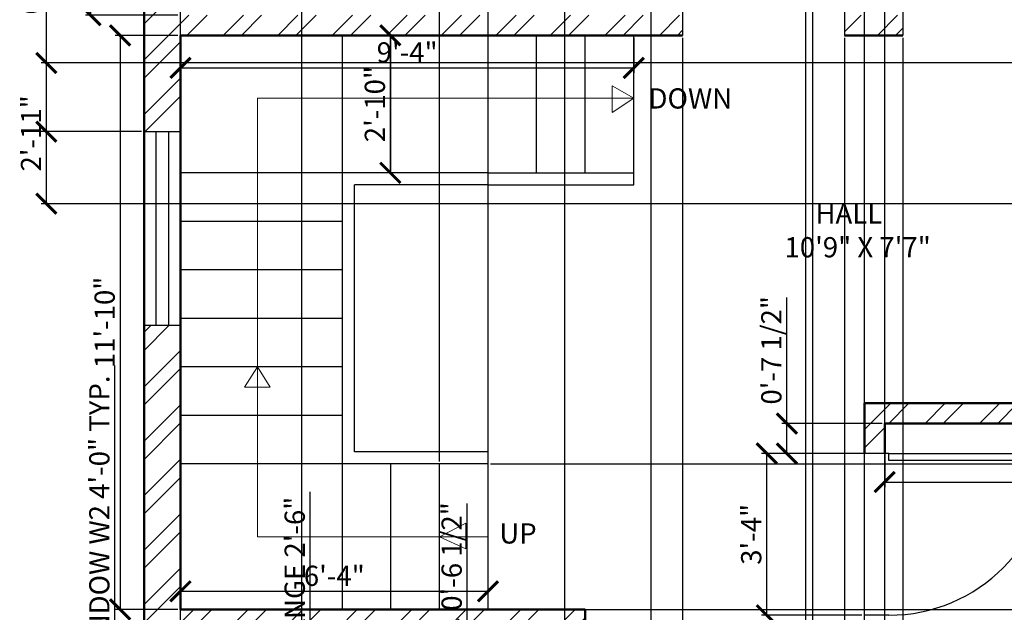
# Model space of a CAD drawing. Units: inches. Extents: x 683 to 1274, y 1901 to 2385.
# Tile 2 of 5: x 687 to 930, y 2049 to 2196. Entities that reach past the tile are written whole.
import ezdxf

# ---------------------------------------------------------------- set-up
doc = ezdxf.new("R2010")
doc.units = ezdxf.units.IN
for name, color, linetype, lineweight in [('A-ANNO-SYMB', 1, 'Continuous', 18), ('A-AREA-IDEN', 3, 'Continuous', 25), ('A-FLOR-STRS', 7, 'Continuous', 25), ('A-WALL-PATT', 8, 'Continuous', 13), ('DIM', 3, 'Continuous', 18), ('DOORS', 4, 'Continuous', 25), ('TEXT', 1, 'Continuous', 25), ('walls', 6, 'Continuous', 50), ('WINDOWS', 30, 'Continuous', 25)]:
    doc.layers.add(name, color=color, linetype=linetype, lineweight=lineweight)
doc.styles.get("Standard").update_dxf_attribs({"font": 'arial.ttf'})
doc.dimstyles.new('ISO-25', dxfattribs={"dimtxt": 5, "dimasz": 5, "dimexe": 1.25, "dimexo": 0.625, "dimtad": 1, "dimdec": 1, "dimlunit": 4, "dimtxsty": 'Standard', "dimblk": 'ARCHTICK', "dimcen": 2.5, "dimadec": 0, "dimazin": 0, "dimtfac": 1, "dimtdec": 1, "dimtmove": 0, "dimatfit": 3, "dimfxl": 1, "dimarcsym": 0})

# ---------------------------------------------------------------- blocks, each defined once
blk = doc.blocks.new('_ArchTick')
at = {"color": 0, "linetype": 'ByBlock', "const_width": 0.15}
blk.add_lwpolyline([(-0.5, -0.5), (0.5, 0.5)], dxfattribs=at)
blk = doc.blocks.new('*D8')
at = {"layer": 'Defpoints', "color": 0, "transparency": 16777216}
for p in [(900.42, 2095.78), (1020.42, 2095.78), (1020.42, 2081.28)]:
    blk.add_point(p, dxfattribs=at)
at = {"layer": 'DIM', "color": 0, "lineweight": -2, "transparency": 16777216}
for p, q in [((900.42, 2095.16), (900.42, 2080.03)), ((1020.42, 2095.16), (1020.42, 2080.03)), ((900.42, 2081.28), (1020.42, 2081.28))]:
    blk.add_line(p, q, dxfattribs=at)
at = {"layer": 'DIM', "color": 0, "lineweight": -2, "transparency": 16777216, "xscale": 5, "yscale": 5, "zscale": 5, "rotation": 180}
blk.add_blockref('_ArchTick', (900.42, 2081.28), dxfattribs=at)
at = {"layer": 'DIM', "color": 0, "lineweight": -2, "transparency": 16777216, "xscale": 5, "yscale": 5, "zscale": 5}
blk.add_blockref('_ArchTick', (1020.42, 2081.28), dxfattribs=at)
at = {"layer": 'DIM', "color": 0, "transparency": 16777216, "insert": (960.42, 2084.46), "char_height": 5, "attachment_point": 5}
blk.add_mtext("10'", dxfattribs=at)
blk = doc.blocks.new('*D12')
at = {"layer": 'Defpoints', "color": 0, "transparency": 16777216}
for p in [(726.42, 2191.78), (838.42, 2191.78), (838.42, 2183.74)]:
    blk.add_point(p, dxfattribs=at)
at = {"layer": 'DIM', "color": 0, "lineweight": -2, "transparency": 16777216}
for p, q in [((726.42, 2191.16), (726.42, 2182.49)), ((838.42, 2191.16), (838.42, 2182.49)), ((726.42, 2183.74), (838.42, 2183.74))]:
    blk.add_line(p, q, dxfattribs=at)
at = {"layer": 'DIM', "color": 0, "lineweight": -2, "transparency": 16777216, "xscale": 5, "yscale": 5, "zscale": 5, "rotation": 180}
blk.add_blockref('_ArchTick', (726.42, 2183.74), dxfattribs=at)
at = {"layer": 'DIM', "color": 0, "lineweight": -2, "transparency": 16777216, "xscale": 5, "yscale": 5, "zscale": 5}
blk.add_blockref('_ArchTick', (838.42, 2183.74), dxfattribs=at)
at = {"layer": 'DIM', "color": 0, "transparency": 16777216, "insert": (782.42, 2186.92), "char_height": 5, "attachment_point": 5}
blk.add_mtext('9\'-4"', dxfattribs=at)
blk = doc.blocks.new('*D13')
at = {"layer": 'Defpoints', "color": 0, "transparency": 16777216}
for p in [(802.42, 2054.27), (726.42, 2049.78), (802.42, 2049.78)]:
    blk.add_point(p, dxfattribs=at)
at = {"layer": 'DIM', "color": 0, "lineweight": -2, "transparency": 16777216}
for p, q in [((726.42, 2050.41), (726.42, 2055.52)), ((726.42, 2054.27), (802.42, 2054.27)), ((802.42, 2050.41), (802.42, 2055.52))]:
    blk.add_line(p, q, dxfattribs=at)
at = {"layer": 'DIM', "color": 0, "lineweight": -2, "transparency": 16777216, "xscale": 5, "yscale": 5, "zscale": 5, "rotation": 180}
blk.add_blockref('_ArchTick', (726.42, 2054.27), dxfattribs=at)
at = {"layer": 'DIM', "color": 0, "lineweight": -2, "transparency": 16777216, "xscale": 5, "yscale": 5, "zscale": 5}
blk.add_blockref('_ArchTick', (802.42, 2054.27), dxfattribs=at)
at = {"layer": 'DIM', "color": 0, "transparency": 16777216, "insert": (764.42, 2057.45), "char_height": 5, "attachment_point": 5}
blk.add_mtext('6\'-4"', dxfattribs=at)
blk = doc.blocks.new('W2')
at = {"layer": 'WINDOWS'}
for p, q in [((1126.75, 2245.25), (1135.75, 2245.25)), ((1126.75, 2197.25), (1126.75, 2245.25)), ((1129.75, 2197.25), (1129.75, 2245.25)), ((1132.75, 2245.25), (1132.75, 2197.25)), ((1135.75, 2245.25), (1135.75, 2197.25)), ((1135.75, 2197.25), (1126.75, 2197.25))]:
    blk.add_line(p, q, dxfattribs=at)
blk = doc.blocks.new('*U18')
for p, q in [((0, 0), (0, -6)), ((40, 0), (40, -6))]:
    blk.add_line(p, q)
blk.add_lwpolyline([(0, 0), (0, 40), (1.75, 40), (1.75, 0)], close=True)
blk.add_arc((0, 0), 40, 0, 90)
blk = doc.blocks.new('*D19')
at = {"layer": 'Defpoints', "color": 0, "transparency": 16777216}
for p in [(726.42, 2328.78), (704.19, 2196.78), (726.42, 2196.78)]:
    blk.add_point(p, dxfattribs=at)
at = {"layer": 'DIM', "color": 0, "lineweight": -2, "transparency": 16777216}
for p, q in [((725.79, 2328.78), (702.94, 2328.78)), ((704.19, 2328.78), (704.19, 2196.78)), ((725.79, 2196.78), (702.94, 2196.78))]:
    blk.add_line(p, q, dxfattribs=at)
at = {"layer": 'DIM', "color": 0, "lineweight": -2, "transparency": 16777216, "xscale": 5, "yscale": 5, "zscale": 5}
for p, rotation in [((704.19, 2328.78), 90), ((704.19, 2196.78), 270)]:
    blk.add_blockref('_ArchTick', p, dxfattribs=dict(at, rotation=rotation))
at = {"layer": 'DIM', "color": 0, "transparency": 16777216, "insert": (701.05, 2262.78), "char_height": 5, "attachment_point": 5, "rotation": 90}
blk.add_mtext("11'", dxfattribs=at)
blk = doc.blocks.new('*D23')
at = {"layer": 'Defpoints', "color": 0, "transparency": 16777216}
for p in [(726.42, 2191.78), (711.49, 2049.78), (726.42, 2049.78)]:
    blk.add_point(p, dxfattribs=at)
at = {"layer": 'DIM', "color": 0, "lineweight": -2, "transparency": 16777216}
for p, q in [((725.79, 2191.78), (710.24, 2191.78)), ((711.49, 2191.78), (711.49, 2049.78)), ((725.79, 2049.78), (710.24, 2049.78))]:
    blk.add_line(p, q, dxfattribs=at)
at = {"layer": 'DIM', "color": 0, "lineweight": -2, "transparency": 16777216, "xscale": 5, "yscale": 5, "zscale": 5}
for p, rotation in [((711.49, 2191.78), 90), ((711.49, 2049.78), 270)]:
    blk.add_blockref('_ArchTick', p, dxfattribs=dict(at, rotation=rotation))
at = {"layer": 'DIM', "color": 0, "transparency": 16777216, "insert": (708.32, 2120.78), "char_height": 5, "attachment_point": 5, "rotation": 90}
blk.add_mtext('11\'-10"', dxfattribs=at)
blk = doc.blocks.new('*D29')
at = {"layer": 'Defpoints', "color": 0, "transparency": 16777216}
for p in [(710.22, 2028.18), (717.42, 2028.18), (717.42, 1980.18)]:
    blk.add_point(p, dxfattribs=at)
at = {"layer": 'DIM', "color": 0, "lineweight": -2, "transparency": 16777216}
for p, q in [((710.22, 2028.18), (710.22, 2110.12)), ((716.79, 2028.18), (708.97, 2028.18)), ((710.22, 1980.18), (710.22, 2028.18)), ((716.79, 1980.18), (708.97, 1980.18))]:
    blk.add_line(p, q, dxfattribs=at)
at = {"layer": 'DIM', "color": 0, "lineweight": -2, "transparency": 16777216, "xscale": 5, "yscale": 5, "zscale": 5}
for p, rotation in [((710.22, 2028.18), 90), ((710.22, 1980.18), 270)]:
    blk.add_blockref('_ArchTick', p, dxfattribs=dict(at, rotation=rotation))
at = {"layer": 'DIM', "color": 0, "transparency": 16777216, "insert": (707.01, 2071.65), "char_height": 5, "attachment_point": 5, "rotation": 90}
blk.add_mtext('WINDOW W2 4\'-0" TYP.', dxfattribs=at)
blk = doc.blocks.new('*D33')
at = {"layer": 'Defpoints', "color": 0, "transparency": 16777216}
for p in [(754, 2032.78), (758.5, 2032.78), (754, 2002.78)]:
    blk.add_point(p, dxfattribs=at)
at = {"layer": 'DIM', "color": 0, "lineweight": -2, "transparency": 16777216}
for p, q in [((758.5, 2032.78), (758.5, 2078.84)), ((754.63, 2032.78), (759.75, 2032.78)), ((758.5, 2002.78), (758.5, 2032.78)), ((754.63, 2002.78), (759.75, 2002.78))]:
    blk.add_line(p, q, dxfattribs=at)
at = {"layer": 'DIM', "color": 0, "lineweight": -2, "transparency": 16777216, "xscale": 5, "yscale": 5, "zscale": 5}
for p, rotation in [((758.5, 2032.78), 90), ((758.5, 2002.78), 270)]:
    blk.add_blockref('_ArchTick', p, dxfattribs=dict(at, rotation=rotation))
at = {"layer": 'DIM', "color": 0, "transparency": 16777216, "insert": (755.29, 2058.31), "char_height": 5, "attachment_point": 5, "rotation": 90}
blk.add_mtext('RANGE 2\'-6"', dxfattribs=at)
blk = doc.blocks.new('*D39')
at = {"layer": 'Defpoints', "color": 0, "transparency": 16777216}
for p in [(900.42, 2361.93), (821.42, 1929.78), (900.42, 1929.78)]:
    blk.add_point(p, dxfattribs=at)
at = {"layer": 'DIM', "color": 0, "lineweight": -2, "transparency": 16777216}
for p, q in [((821.42, 1930.41), (821.42, 2363.18)), ((900.42, 1930.41), (900.42, 2363.18)), ((821.42, 2361.93), (900.42, 2361.93))]:
    blk.add_line(p, q, dxfattribs=at)
at = {"layer": 'DIM', "color": 0, "lineweight": -2, "transparency": 16777216, "xscale": 5, "yscale": 5, "zscale": 5, "rotation": 180}
blk.add_blockref('_ArchTick', (821.42, 2361.93), dxfattribs=at)
at = {"layer": 'DIM', "color": 0, "lineweight": -2, "transparency": 16777216, "xscale": 5, "yscale": 5, "zscale": 5}
blk.add_blockref('_ArchTick', (900.42, 2361.93), dxfattribs=at)
at = {"layer": 'DIM', "color": 0, "transparency": 16777216, "insert": (860.92, 2365.11), "char_height": 5, "attachment_point": 5}
blk.add_mtext('6\'-7"', dxfattribs=at)
blk = doc.blocks.new('*D43')
at = {"layer": 'Defpoints', "color": 0, "transparency": 16777216}
for p in [(693.27, 2184.95), (967.42, 2184.95), (967.42, 2150.14)]:
    blk.add_point(p, dxfattribs=at)
at = {"layer": 'DIM', "color": 0, "lineweight": -2, "transparency": 16777216}
for p, q in [((966.79, 2184.95), (692.02, 2184.95)), ((693.27, 2150.14), (693.27, 2184.95)), ((966.79, 2150.14), (692.02, 2150.14))]:
    blk.add_line(p, q, dxfattribs=at)
at = {"layer": 'DIM', "color": 0, "lineweight": -2, "transparency": 16777216, "xscale": 5, "yscale": 5, "zscale": 5}
for p, rotation in [((693.27, 2184.95), 90), ((693.27, 2150.14), 270)]:
    blk.add_blockref('_ArchTick', p, dxfattribs=dict(at, rotation=rotation))
at = {"layer": 'DIM', "color": 0, "transparency": 16777216, "insert": (690.13, 2167.54), "char_height": 5, "attachment_point": 5, "rotation": 90}
blk.add_mtext('2\'-11"', dxfattribs=at)
blk = doc.blocks.new('*D44')
at = {"layer": 'Defpoints', "color": 0, "transparency": 16777216}
for p in [(882.7, 2361.93), (842.7, 1953.78), (882.7, 1953.78)]:
    blk.add_point(p, dxfattribs=at)
at = {"layer": 'DIM', "color": 0, "lineweight": -2, "transparency": 16777216}
for p, q in [((842.7, 1954.41), (842.7, 2363.18)), ((882.7, 1954.41), (882.7, 2363.18)), ((842.7, 2361.93), (882.7, 2361.93))]:
    blk.add_line(p, q, dxfattribs=at)
at = {"layer": 'DIM', "color": 0, "lineweight": -2, "transparency": 16777216, "xscale": 5, "yscale": 5, "zscale": 5, "rotation": 180}
blk.add_blockref('_ArchTick', (842.7, 2361.93), dxfattribs=at)
at = {"layer": 'DIM', "color": 0, "lineweight": -2, "transparency": 16777216, "xscale": 5, "yscale": 5, "zscale": 5}
blk.add_blockref('_ArchTick', (882.7, 2361.93), dxfattribs=at)
at = {"layer": 'DIM', "color": 0, "transparency": 16777216, "insert": (862.7, 2365.11), "char_height": 5, "attachment_point": 5}
blk.add_mtext('3\'-4"', dxfattribs=at)
blk = doc.blocks.new('*D45')
at = {"layer": 'Defpoints', "color": 0, "transparency": 16777216}
for p in [(850.48, 2191.78), (890.48, 2191.78), (890.48, 1905.63)]:
    blk.add_point(p, dxfattribs=at)
at = {"layer": 'DIM', "color": 0, "lineweight": -2, "transparency": 16777216}
for p, q in [((850.48, 2191.16), (850.48, 1904.38)), ((890.48, 2191.16), (890.48, 1904.38)), ((850.48, 1905.63), (890.48, 1905.63))]:
    blk.add_line(p, q, dxfattribs=at)
at = {"layer": 'DIM', "color": 0, "lineweight": -2, "transparency": 16777216, "xscale": 5, "yscale": 5, "zscale": 5, "rotation": 180}
blk.add_blockref('_ArchTick', (850.48, 1905.63), dxfattribs=at)
at = {"layer": 'DIM', "color": 0, "lineweight": -2, "transparency": 16777216, "xscale": 5, "yscale": 5, "zscale": 5}
blk.add_blockref('_ArchTick', (890.48, 1905.63), dxfattribs=at)
at = {"layer": 'DIM', "color": 0, "transparency": 16777216, "insert": (870.48, 1908.81), "char_height": 5, "attachment_point": 5}
blk.add_mtext('3\'-4"', dxfattribs=at)
blk = doc.blocks.new('*D46')
at = {"layer": 'Defpoints', "color": 0, "transparency": 16777216}
for p in [(904.89, 2191.78), (944.89, 2191.78), (944.89, 1905.63)]:
    blk.add_point(p, dxfattribs=at)
at = {"layer": 'DIM', "color": 0, "lineweight": -2, "transparency": 16777216}
for p, q in [((904.89, 2191.16), (904.89, 1904.38)), ((944.89, 2191.16), (944.89, 1904.38)), ((904.89, 1905.63), (944.89, 1905.63))]:
    blk.add_line(p, q, dxfattribs=at)
at = {"layer": 'DIM', "color": 0, "lineweight": -2, "transparency": 16777216, "xscale": 5, "yscale": 5, "zscale": 5, "rotation": 180}
blk.add_blockref('_ArchTick', (904.89, 1905.63), dxfattribs=at)
at = {"layer": 'DIM', "color": 0, "lineweight": -2, "transparency": 16777216, "xscale": 5, "yscale": 5, "zscale": 5}
blk.add_blockref('_ArchTick', (944.89, 1905.63), dxfattribs=at)
at = {"layer": 'DIM', "color": 0, "transparency": 16777216, "insert": (924.89, 1908.81), "char_height": 5, "attachment_point": 5}
blk.add_mtext('3\'-4"', dxfattribs=at)
blk = doc.blocks.new('*D47')
at = {"layer": 'Defpoints', "color": 0, "transparency": 16777216}
for p in [(871.27, 2088.36), (895.42, 2088.36), (895.42, 2048.36)]:
    blk.add_point(p, dxfattribs=at)
at = {"layer": 'DIM', "color": 0, "lineweight": -2, "transparency": 16777216}
for p, q in [((894.79, 2088.36), (870.02, 2088.36)), ((871.27, 2048.36), (871.27, 2088.36)), ((894.79, 2048.36), (870.02, 2048.36))]:
    blk.add_line(p, q, dxfattribs=at)
at = {"layer": 'DIM', "color": 0, "lineweight": -2, "transparency": 16777216, "xscale": 5, "yscale": 5, "zscale": 5}
for p, rotation in [((871.27, 2088.36), 90), ((871.27, 2048.36), 270)]:
    blk.add_blockref('_ArchTick', p, dxfattribs=dict(at, rotation=rotation))
at = {"layer": 'DIM', "color": 0, "transparency": 16777216, "insert": (868.09, 2068.36), "char_height": 5, "attachment_point": 5, "rotation": 90}
blk.add_mtext('3\'-4"', dxfattribs=at)
blk = doc.blocks.new('*D48')
at = {"layer": 'Defpoints', "color": 0, "transparency": 16777216}
for p in [(778.27, 2191.78), (802.42, 2191.78), (802.42, 2157.78)]:
    blk.add_point(p, dxfattribs=at)
at = {"layer": 'DIM', "color": 0, "lineweight": -2, "transparency": 16777216}
for p, q in [((801.79, 2191.78), (777.02, 2191.78)), ((778.27, 2157.78), (778.27, 2191.78)), ((801.79, 2157.78), (777.02, 2157.78))]:
    blk.add_line(p, q, dxfattribs=at)
at = {"layer": 'DIM', "color": 0, "lineweight": -2, "transparency": 16777216, "xscale": 5, "yscale": 5, "zscale": 5}
for p, rotation in [((778.27, 2191.78), 90), ((778.27, 2157.78), 270)]:
    blk.add_blockref('_ArchTick', p, dxfattribs=dict(at, rotation=rotation))
at = {"layer": 'DIM', "color": 0, "transparency": 16777216, "insert": (775.09, 2174.78), "char_height": 5, "attachment_point": 5, "rotation": 90}
blk.add_mtext('2\'-10"', dxfattribs=at)
blk = doc.blocks.new('*D49')
at = {"layer": 'Defpoints', "color": 0, "transparency": 16777216}
for p in [(802.42, 2085.78), (1053.57, 2085.78), (802.42, 2049.78)]:
    blk.add_point(p, dxfattribs=at)
at = {"layer": 'DIM', "color": 0, "lineweight": -2, "transparency": 16777216}
for p, q in [((803.04, 2085.78), (1054.82, 2085.78)), ((1053.57, 2049.78), (1053.57, 2085.78)), ((803.04, 2049.78), (1054.82, 2049.78))]:
    blk.add_line(p, q, dxfattribs=at)
at = {"layer": 'DIM', "color": 0, "lineweight": -2, "transparency": 16777216, "xscale": 5, "yscale": 5, "zscale": 5}
for p, rotation in [((1053.57, 2085.78), 90), ((1053.57, 2049.78), 270)]:
    blk.add_blockref('_ArchTick', p, dxfattribs=dict(at, rotation=rotation))
at = {"layer": 'DIM', "color": 0, "transparency": 16777216, "insert": (1050.39, 2067.78), "char_height": 5, "attachment_point": 5, "rotation": 90}
blk.add_mtext('3\'-0"', dxfattribs=at)
blk = doc.blocks.new('*D50')
at = {"layer": 'Defpoints', "color": 0, "transparency": 16777216}
for p in [(802.42, 2361.93), (790.42, 2085.78), (802.42, 2085.78)]:
    blk.add_point(p, dxfattribs=at)
at = {"layer": 'DIM', "color": 0, "lineweight": -2, "transparency": 16777216}
for p, q in [((790.42, 2086.41), (790.42, 2363.18)), ((802.42, 2086.41), (802.42, 2363.18)), ((790.42, 2361.93), (802.42, 2361.93)), ((802.42, 2361.93), (821.49, 2361.93))]:
    blk.add_line(p, q, dxfattribs=at)
at = {"layer": 'DIM', "color": 0, "lineweight": -2, "transparency": 16777216, "xscale": 5, "yscale": 5, "zscale": 5, "rotation": 180}
blk.add_blockref('_ArchTick', (790.42, 2361.93), dxfattribs=at)
at = {"layer": 'DIM', "color": 0, "lineweight": -2, "transparency": 16777216, "xscale": 5, "yscale": 5, "zscale": 5}
blk.add_blockref('_ArchTick', (802.42, 2361.93), dxfattribs=at)
at = {"layer": 'DIM', "color": 0, "transparency": 16777216, "insert": (814.45, 2365.11), "char_height": 5, "attachment_point": 5}
blk.add_mtext('1\'-0"', dxfattribs=at)
blk = doc.blocks.new('*D55')
at = {"layer": 'Defpoints', "color": 0, "transparency": 16777216}
for p in [(693.27, 2240.95), (717.42, 2240.95), (717.42, 2167.98)]:
    blk.add_point(p, dxfattribs=at)
at = {"layer": 'DIM', "color": 0, "lineweight": -2, "transparency": 16777216}
for p, q in [((716.79, 2240.95), (692.02, 2240.95)), ((693.27, 2167.98), (693.27, 2240.95)), ((716.79, 2167.98), (692.02, 2167.98))]:
    blk.add_line(p, q, dxfattribs=at)
at = {"layer": 'DIM', "color": 0, "lineweight": -2, "transparency": 16777216, "xscale": 5, "yscale": 5, "zscale": 5}
for p, rotation in [((693.27, 2240.95), 90), ((693.27, 2167.98), 270)]:
    blk.add_blockref('_ArchTick', p, dxfattribs=dict(at, rotation=rotation))
at = {"layer": 'DIM', "color": 0, "transparency": 16777216, "insert": (690.09, 2204.46), "char_height": 5, "attachment_point": 5, "rotation": 90}
blk.add_mtext('6\'-1"', dxfattribs=at)
blk = doc.blocks.new('*D58')
at = {"layer": 'Defpoints', "color": 0, "transparency": 16777216}
for p in [(756.42, 2361.93), (726.42, 2044.78), (756.42, 2044.78)]:
    blk.add_point(p, dxfattribs=at)
at = {"layer": 'DIM', "color": 0, "lineweight": -2, "transparency": 16777216}
for p, q in [((726.42, 2045.41), (726.42, 2363.18)), ((756.42, 2045.41), (756.42, 2363.18)), ((726.42, 2361.93), (756.42, 2361.93))]:
    blk.add_line(p, q, dxfattribs=at)
at = {"layer": 'DIM', "color": 0, "lineweight": -2, "transparency": 16777216, "xscale": 5, "yscale": 5, "zscale": 5, "rotation": 180}
blk.add_blockref('_ArchTick', (726.42, 2361.93), dxfattribs=at)
at = {"layer": 'DIM', "color": 0, "lineweight": -2, "transparency": 16777216, "xscale": 5, "yscale": 5, "zscale": 5}
blk.add_blockref('_ArchTick', (756.42, 2361.93), dxfattribs=at)
at = {"layer": 'DIM', "color": 0, "transparency": 16777216, "insert": (741.42, 2365.11), "char_height": 5, "attachment_point": 5}
blk.add_mtext('2\'-6"', dxfattribs=at)
blk = doc.blocks.new('*D61')
at = {"layer": 'Defpoints', "color": 0, "transparency": 16777216}
for p in [(895.42, 2361.93), (880.95, 1962.78), (895.42, 1962.78)]:
    blk.add_point(p, dxfattribs=at)
at = {"layer": 'DIM', "color": 0, "lineweight": -2, "transparency": 16777216}
for p, q in [((880.95, 1963.41), (880.95, 2363.18)), ((895.42, 1963.41), (895.42, 2363.18)), ((880.95, 2361.93), (895.42, 2361.93)), ((895.42, 2361.93), (926.14, 2361.93))]:
    blk.add_line(p, q, dxfattribs=at)
at = {"layer": 'DIM', "color": 0, "lineweight": -2, "transparency": 16777216, "xscale": 5, "yscale": 5, "zscale": 5, "rotation": 180}
blk.add_blockref('_ArchTick', (880.95, 2361.93), dxfattribs=at)
at = {"layer": 'DIM', "color": 0, "lineweight": -2, "transparency": 16777216, "xscale": 5, "yscale": 5, "zscale": 5}
blk.add_blockref('_ArchTick', (895.42, 2361.93), dxfattribs=at)
at = {"layer": 'DIM', "color": 0, "transparency": 16777216, "insert": (913.28, 2365.14), "char_height": 5, "attachment_point": 5}
blk.add_mtext('1\'-2 1/2"', dxfattribs=at)
blk = doc.blocks.new('*D65')
at = {"layer": 'Defpoints', "color": 0, "transparency": 16777216}
for p in [(876.27, 2095.78), (900.42, 2095.78), (900.42, 2088.36)]:
    blk.add_point(p, dxfattribs=at)
at = {"layer": 'DIM', "color": 0, "lineweight": -2, "transparency": 16777216}
for p, q in [((876.27, 2095.78), (876.27, 2126.97)), ((899.79, 2095.78), (875.02, 2095.78)), ((876.27, 2088.36), (876.27, 2095.78)), ((899.79, 2088.36), (875.02, 2088.36))]:
    blk.add_line(p, q, dxfattribs=at)
at = {"layer": 'DIM', "color": 0, "lineweight": -2, "transparency": 16777216, "xscale": 5, "yscale": 5, "zscale": 5}
for p, rotation in [((876.27, 2095.78), 90), ((876.27, 2088.36), 270)]:
    blk.add_blockref('_ArchTick', p, dxfattribs=dict(at, rotation=rotation))
at = {"layer": 'DIM', "color": 0, "transparency": 16777216, "insert": (873.06, 2113.88), "char_height": 5, "attachment_point": 5, "rotation": 90}
blk.add_mtext('0\'-7 1/2"', dxfattribs=at)
blk = doc.blocks.new('*D66')
at = {"layer": 'Defpoints', "color": 0, "transparency": 16777216}
for p in [(797.27, 2044.78), (821.42, 2044.78), (821.42, 2038.04)]:
    blk.add_point(p, dxfattribs=at)
at = {"layer": 'DIM', "color": 0, "lineweight": -2, "transparency": 16777216}
for p, q in [((797.27, 2044.78), (797.27, 2075.97)), ((820.79, 2044.78), (796.02, 2044.78)), ((797.27, 2038.04), (797.27, 2044.78)), ((820.79, 2038.04), (796.02, 2038.04))]:
    blk.add_line(p, q, dxfattribs=at)
at = {"layer": 'DIM', "color": 0, "lineweight": -2, "transparency": 16777216, "xscale": 5, "yscale": 5, "zscale": 5}
for p, rotation in [((797.27, 2044.78), 90), ((797.27, 2038.04), 270)]:
    blk.add_blockref('_ArchTick', p, dxfattribs=dict(at, rotation=rotation))
at = {"layer": 'DIM', "color": 0, "transparency": 16777216, "insert": (794.06, 2062.88), "char_height": 5, "attachment_point": 5, "rotation": 90}
blk.add_mtext('0\'-6 1/2"', dxfattribs=at)

msp = doc.modelspace()

# ---------------------------------------------------------------- hatches: boundary and pattern name
at = {"layer": 'A-WALL-PATT'}
h = msp.add_hatch(dxfattribs=at)
h.set_pattern_fill('ANSI32', color=256)
h.paths.add_polyline_path([(717.42, 2337.78), (717.42, 2300.95), (726.42, 2300.95), (726.42, 2328.78), (895.42, 2328.78), (895.42, 2196.78), (890.48, 2196.78), (890.48, 2191.78), (904.89, 2191.78), (904.89, 2196.78), (900.42, 2196.78), (900.42, 2328.78), (1020.42, 2328.78), (1020.42, 2303.09), (1029.42, 2303.09), (1029.42, 2337.78)])
h.paths.add_polyline_path([(1020.42, 2196.78), (944.89, 2196.78), (944.89, 2191.78), (967.42, 2191.78), (967.42, 2184.95), (972.42, 2184.95), (972.42, 2191.78), (1020.42, 2191.78), (1020.42, 2129.51), (1029.42, 2129.51), (1029.42, 2243.09), (1020.42, 2243.09)])
h.paths.add_polyline_path([(1029.42, 2105.51), (1020.42, 2105.51), (1020.42, 2100.78), (972.42, 2100.78), (972.42, 2150.14), (967.42, 2150.14), (967.42, 2100.78), (895.42, 2100.78), (895.42, 2088.36), (900.42, 2088.36), (900.42, 2095.78), (1020.42, 2095.78), (1020.42, 1962.78), (1000.32, 1962.78), (1000.32, 1953.78), (1029.42, 1953.78)])
h.paths.add_polyline_path([(940.32, 1953.78), (940.32, 1962.78), (900.42, 1962.78), (900.42, 2048.36), (895.42, 2048.36), (895.42, 1962.78), (882.7, 1962.78), (882.7, 1959.78), (882.7, 1953.78)])
h.paths.add_polyline_path([(790.86, 1953.78), (790.86, 1962.78), (726.42, 1962.78), (726.42, 1980.18), (717.42, 1980.18), (717.42, 1953.78)])
h.paths.add_polyline_path([(842.7, 1953.78), (842.7, 1959.78, -0.01877), (842.81, 1962.78), (826.42, 1962.78), (826.42, 2003.23), (821.42, 2003.23), (821.42, 1962.78), (814.86, 1962.78), (814.86, 1953.78)])
h.paths.add_polyline_path([(726.42, 2196.78), (726.42, 2240.95), (717.42, 2240.95), (717.42, 2167.98), (726.42, 2167.98), (726.42, 2191.78), (850.48, 2191.78), (850.48, 2196.78)])
h = msp.add_hatch(dxfattribs=at)
h.set_pattern_fill('ANSI32', color=256)
h.paths.add_polyline_path([(726.42, 2119.98), (717.42, 2119.98), (717.42, 2028.18), (726.42, 2028.18), (726.42, 2044.78), (821.42, 2044.78), (821.42, 2038.04), (826.42, 2038.04), (826.42, 2049.78), (726.42, 2049.78)])

# ---------------------------------------------------------------- linework, layer by layer
at = {"layer": 'A-ANNO-SYMB'}
for p, q in [((838.42, 2176.26), (833.12, 2179.34)), ((833.12, 2179.34), (833.12, 2172.74)), ((745.43, 2067.78), (745.43, 2176.26)), ((745.43, 2176.26), (838.42, 2176.26)), ((833.12, 2172.74), (838.42, 2176.26)), ((745.43, 2109.78), (742.27, 2104.8)), ((748.59, 2104.8), (745.43, 2109.78)), ((742.27, 2104.8), (748.59, 2104.8)), ((790.42, 2067.78), (796.96, 2071.1)), ((796.96, 2071.1), (796.96, 2064.74)), ((802.42, 2067.78), (745.43, 2067.78)), ((796.96, 2064.74), (790.42, 2067.78))]:
    msp.add_line(p, q, dxfattribs=at)
at = {"layer": 'A-FLOR-STRS'}
for p, q in [((766.42, 2085.78), (766.42, 2191.78)), ((778.42, 2157.78), (778.42, 2191.78)), ((790.42, 2157.78), (790.42, 2191.78)), ((802.42, 2157.78), (802.42, 2191.78)), ((814.42, 2157.78), (814.42, 2191.78)), ((826.42, 2157.78), (826.42, 2191.78)), ((838.42, 2154.78), (838.42, 2191.78)), ((802.42, 2157.78), (726.42, 2157.78)), ((802.42, 2157.78), (838.42, 2157.78)), ((769.42, 2088.78), (769.42, 2154.78)), ((802.42, 2154.78), (769.42, 2154.78)), ((802.42, 2154.78), (838.42, 2154.78)), ((766.42, 2145.78), (726.42, 2145.78)), ((766.42, 2133.78), (726.42, 2133.78)), ((766.42, 2121.78), (726.42, 2121.78)), ((766.42, 2109.78), (726.42, 2109.78)), ((766.42, 2097.78), (726.42, 2097.78)), ((802.42, 2088.78), (769.42, 2088.78)), ((802.42, 2085.78), (802.42, 2088.78)), ((802.42, 2085.78), (802.42, 2088.78)), ((802.42, 2085.78), (726.42, 2085.78)), ((766.42, 2049.78), (766.42, 2085.78)), ((778.42, 2049.78), (778.42, 2085.78)), ((790.42, 2049.78), (790.42, 2085.78)), ((802.42, 2049.78), (802.42, 2085.78))]:
    msp.add_line(p, q, dxfattribs=at)
at = {"layer": 'walls'}
for p, q in [((717.42, 2337.78), (717.42, 1953.78)), ((726.42, 2191.78), (850.48, 2191.78)), ((726.42, 2191.78), (726.42, 2049.78)), ((890.48, 2191.78), (904.89, 2191.78)), ((895.42, 2100.78), (967.42, 2100.78)), ((895.42, 2100.78), (895.42, 2088.36)), ((900.42, 2095.78), (900.42, 2088.36)), ((900.42, 2095.78), (1020.42, 2095.78)), ((826.42, 2049.78), (726.42, 2049.78)), ((826.42, 2038.04), (826.42, 2049.78))]:
    msp.add_line(p, q, dxfattribs=at)

# ---------------------------------------------------------------- block references
at = {"layer": 'DOORS', "xscale": -1}
msp.add_blockref('*U18', (890.48, 2197.78), dxfattribs=at)
at = {"layer": 'DOORS'}
msp.add_blockref('*U18', (904.89, 2197.78), dxfattribs=at)
at = {"layer": 'DOORS', "rotation": 270}
msp.add_blockref('*U18', (901.42, 2088.36), dxfattribs=at)
at = {"layer": 'WINDOWS'}
msp.add_blockref('W2', (-409.33, -77.27), dxfattribs=at)

# ---------------------------------------------------------------- texts
at = {"layer": 'A-AREA-IDEN', "insert": (875.66, 2150.21), "char_height": 5, "attachment_point": 1}
msp.add_mtext_dynamic_manual_height_columns('{     HALL\\P10\'9" X 7\'7"}', width=38.5091, gutter_width=12.5, heights=[0], dxfattribs=at)
at = {"layer": 'TEXT', "char_height": 5, "attachment_point": 1}
for s, insert in [('{DOWN}', (842.06, 2178.68)), ('{UP}', (805.19, 2071.09))]:
    msp.add_mtext_dynamic_manual_height_columns(s, width=7.8955, gutter_width=12.5, heights=[0], dxfattribs=dict(at, insert=insert))

# ---------------------------------------------------------------- dimensions: what is measured, and where the dimension line sits
at = {"layer": 'DIM'}
for base, p1, p2, override, picture, middle in [((895.42, 2361.93), (880.95, 1962.78), (895.42, 1962.78), {"dimdec": 1, "dimlfac": 1, "dimrnd": 0, "dimzin": 1, "dimdsep": 46, "dimlunit": 4, "dimfrac": 2}, '*D61', (913.28, 2365.14)), ((756.42, 2361.93), (726.42, 2044.78), (756.42, 2044.78), {"dimdec": 1, "dimlfac": 1, "dimrnd": 0, "dimzin": 1, "dimdsep": 46, "dimlunit": 4, "dimfrac": 2}, '*D58', (741.42, 2365.11)), ((802.42, 2361.93), (790.42, 2085.78), (802.42, 2085.78), {"dimdec": 1, "dimlfac": 1, "dimrnd": 0, "dimzin": 1, "dimdsep": 46, "dimlunit": 4, "dimfrac": 2}, '*D50', (814.45, 2365.11)), ((900.42, 2361.93), (821.42, 1929.78), (900.42, 1929.78), {"dimdec": 1, "dimlfac": 1, "dimrnd": 0, "dimzin": 1, "dimdsep": 46, "dimlunit": 4, "dimfrac": 2}, '*D39', (860.92, 2365.11)), ((882.7, 2361.93), (842.7, 1953.78), (882.7, 1953.78), {"dimdec": 1, "dimlfac": 1, "dimrnd": 0, "dimzin": 1, "dimdsep": 46, "dimlunit": 4, "dimfrac": 2}, '*D44', (862.7, 2365.11)), ((838.42, 2183.74), (726.42, 2191.78), (838.42, 2191.78), {"dimclrd": 0, "dimclre": 0, "dimclrt": 0}, '*D12', (782.42, 2186.92)), ((890.48, 1905.63), (850.48, 2191.78), (890.48, 2191.78), {"dimdec": 1, "dimlfac": 1, "dimrnd": 0, "dimzin": 1, "dimdsep": 46, "dimlunit": 4, "dimfrac": 2}, '*D45', (870.48, 1908.81)), ((944.89, 1905.63), (904.89, 2191.78), (944.89, 2191.78), {"dimdec": 1, "dimlfac": 1, "dimrnd": 0, "dimzin": 1, "dimdsep": 46, "dimlunit": 4, "dimfrac": 2}, '*D46', (924.89, 1908.81)), ((1020.42, 2081.28), (900.42, 2095.78), (1020.42, 2095.78), {"dimclrd": 0, "dimclre": 0, "dimclrt": 0}, '*D8', (960.42, 2084.46)), ((802.42, 2054.27), (726.42, 2049.78), (802.42, 2049.78), {"dimclrd": 0, "dimclre": 0, "dimclrt": 0}, '*D13', (764.42, 2057.45))]:
    dim = msp.add_linear_dim(base=base, p1=p1, p2=p2, dimstyle='ISO-25', override=override, dxfattribs=at)
    dim.commit()
    dim.dimension.update_dxf_attribs({"geometry": picture, "text_midpoint": middle})
for base, p1, p2, override, picture, middle in [((704.19, 2196.78), (726.42, 2328.78), (726.42, 2196.78), {"dimclrd": 0, "dimclre": 0, "dimclrt": 0}, '*D19', (701.05, 2262.78)), ((693.27, 2240.95), (717.42, 2167.98), (717.42, 2240.95), {"dimdec": 1, "dimlfac": 1, "dimrnd": 0, "dimzin": 1, "dimdsep": 46, "dimlunit": 4, "dimfrac": 2}, '*D55', (690.09, 2204.46)), ((711.49, 2049.78), (726.42, 2191.78), (726.42, 2049.78), {"dimclrd": 0, "dimclre": 0, "dimclrt": 0}, '*D23', (708.32, 2120.78)), ((778.27, 2191.78), (802.42, 2157.78), (802.42, 2191.78), {"dimdec": 1, "dimlfac": 1, "dimrnd": 0, "dimzin": 1, "dimdsep": 46, "dimlunit": 4, "dimfrac": 2}, '*D48', (775.09, 2174.78)), ((693.27, 2184.95), (967.42, 2150.14), (967.42, 2184.95), {"dimdec": 1, "dimlfac": 1, "dimrnd": 0, "dimzin": 1, "dimdsep": 46, "dimlunit": 4, "dimfrac": 2}, '*D43', (690.13, 2167.54)), ((876.27, 2095.78), (900.42, 2088.36), (900.42, 2095.78), {"dimdec": 1, "dimlfac": 1, "dimrnd": 0, "dimzin": 1, "dimdsep": 46, "dimlunit": 4, "dimfrac": 2}, '*D65', (873.06, 2113.88)), ((871.27, 2088.36), (895.42, 2048.36), (895.42, 2088.36), {"dimdec": 1, "dimlfac": 1, "dimrnd": 0, "dimzin": 1, "dimdsep": 46, "dimlunit": 4, "dimfrac": 2}, '*D47', (868.09, 2068.36)), ((1053.57, 2085.78), (802.42, 2049.78), (802.42, 2085.78), {"dimdec": 1, "dimlfac": 1, "dimrnd": 0, "dimzin": 1, "dimdsep": 46, "dimlunit": 4, "dimfrac": 2}, '*D49', (1050.39, 2067.78)), ((797.27, 2044.78), (821.42, 2038.04), (821.42, 2044.78), {"dimdec": 1, "dimlfac": 1, "dimrnd": 0, "dimzin": 1, "dimdsep": 46, "dimlunit": 4, "dimfrac": 2}, '*D66', (794.06, 2062.88))]:
    dim = msp.add_linear_dim(base=base, p1=p1, p2=p2, angle=90, dimstyle='ISO-25', override=override, dxfattribs=at)
    dim.commit()
    dim.dimension.update_dxf_attribs({"geometry": picture, "text_midpoint": middle})
for base, p1, p2, text, picture, middle in [((710.22, 2028.18), (717.42, 1980.18), (717.42, 2028.18), 'WINDOW W2 <> TYP.', '*D29', (707.01, 2071.65)), ((758.5, 2032.78), (754, 2002.78), (754, 2032.78), 'RANGE <>', '*D33', (755.29, 2058.31))]:
    dim = msp.add_linear_dim(base=base, p1=p1, p2=p2, angle=90, text=text, dimstyle='ISO-25', override={"dimdec": 1, "dimlfac": 1, "dimrnd": 0, "dimzin": 1, "dimdsep": 46, "dimlunit": 4, "dimfrac": 2}, dxfattribs=at)
    dim.commit()
    dim.dimension.update_dxf_attribs({"geometry": picture, "text_midpoint": middle})

doc.saveas('drawing.dxf')
